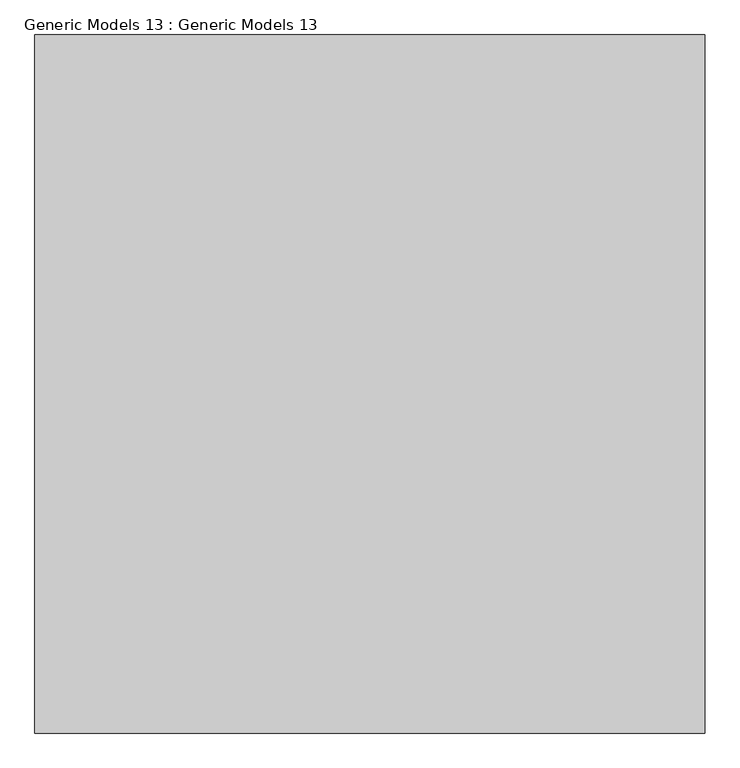
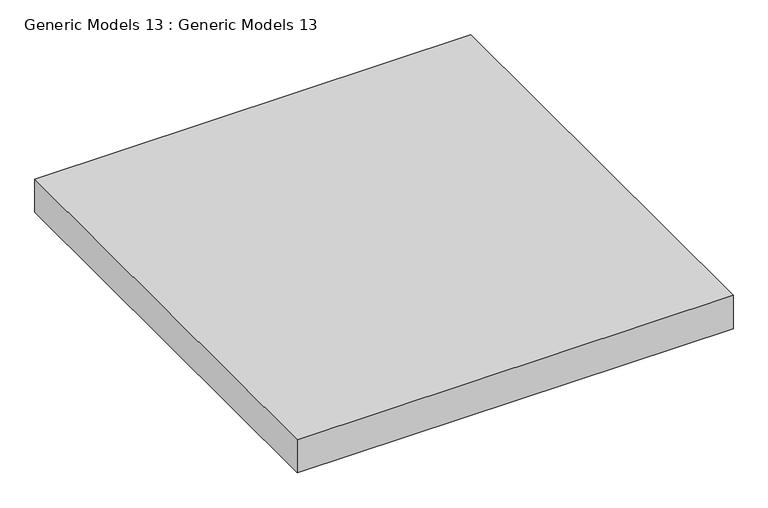
"""IFC4 building model written with IfcOpenShell, lengths in millimetres: proxy geometry, Generic Models 13 : Generic Models 13."""

from ifc_helpers import new_model, si_unit, frame, origin, place, context, project, spatial, polyline, outline, extrude, source, transform, mapped, element, save


def generic_models_13_generic_models_13_5b4bef59(model_context):
    return source(origin(), model_context, "Body", "SweptSolid", [
        extrude(outline(polyline([(16213.1169441, 17574.6572885), (16213.1169441, -13715.6423762), (-13833.4638778, -13715.6423762), (-13833.4638778, 17574.6572885), (16213.1169441, 17574.6572885)])), frame((0.0, 0.0, 18918.7849443), z_axis=(0.0, 0.0, 1.0), x_axis=(1.0, 0.0, 0.0)), (0.0, 0.0, 1.0), 2415.2962908),
    ])


if __name__ == "__main__":
    model = new_model("IFC4")
    model_context = context("Model", 3, world=origin())
    ifc_project = project(units=[si_unit("LENGTHUNIT", "METRE", prefix="MILLI")], contexts=[model_context])
    site = spatial("IfcSite", under=ifc_project)
    building = spatial("IfcBuilding", under=site)
    placement = place(None, origin())
    generic_models_13_generic_models_13_shape = generic_models_13_generic_models_13_5b4bef59(model_context)
    element("IfcBuildingElementProxy", 1, Name="Generic Models 13 : Generic Models 13", ObjectType="Generic Models 13 : Generic Models 13", at=placement, inside=building, context=model_context, shape_type="MappedRepresentation", body=[
        mapped(generic_models_13_generic_models_13_shape, transform((0.0, 0.0, 0.0), x_axis=(1.0, 0.0, 0.0), y_axis=(0.0, 1.0, 0.0), z_axis=(0.0, 0.0, 1.0))),
    ])
    save(model, "model.ifc")
